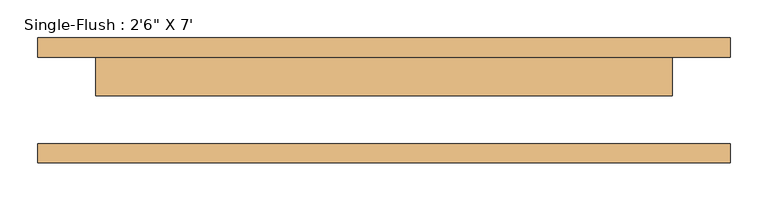
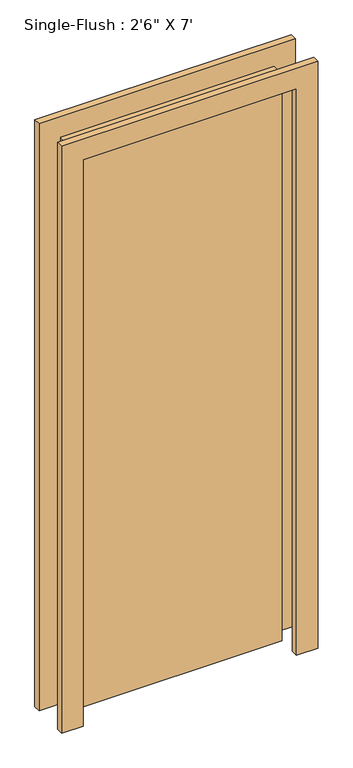
"""IFC4 building model written with IfcOpenShell, lengths in millimetres: door geometry."""

from ifc_helpers import new_model, si_unit, frame, origin, origin_with_axes, place, context, project, spatial, polyline, outline, extrude, source, transform, mapped, element, save


def door_214872d5(model_context):
    return source(origin(), model_context, "Body", "SweptSolid", [
        extrude(outline(polyline([(2209.8, -457.2), (0.0, -457.2), (0.0, -381.0), (2133.6, -381.0), (2133.6, 381.0), (0.0, 381.0), (0.0, 457.2), (2209.8, 457.2), (2209.8, -457.2)])), frame((0.0, 57.15, 0.0), z_axis=(0.0, 1.0, 0.0), x_axis=(0.0, 0.0, 1.0)), (0.0, 0.0, 1.0), 25.4),
        extrude(outline(polyline([(2209.8, 457.2), (2209.8, -457.2), (0.0, -457.2), (0.0, -381.0), (2133.6, -381.0), (2133.6, 381.0), (0.0, 381.0), (0.0, 457.2), (2209.8, 457.2)])), frame((0.0, -82.55, 0.0), z_axis=(0.0, 1.0, 0.0), x_axis=(0.0, 0.0, 1.0)), (0.0, 0.0, 1.0), 25.4),
        extrude(outline(polyline([(381.0, 6.35), (-381.0, 6.35), (-381.0, 57.15), (381.0, 57.15), (381.0, 6.35)])), origin_with_axes(), (0.0, 0.0, 1.0), 2133.6),
    ])


if __name__ == "__main__":
    model = new_model("IFC4")
    model_context = context("Model", 3, world=origin())
    ifc_project = project(units=[si_unit("LENGTHUNIT", "METRE", prefix="MILLI")], contexts=[model_context])
    site = spatial("IfcSite", under=ifc_project)
    building = spatial("IfcBuilding", under=site)
    placement = place(None, origin())
    door_shape = door_214872d5(model_context)
    element("IfcDoor", 1, ObjectType="Single-Flush : 2'6\" X 7'", at=placement, inside=building, context=model_context, shape_type="MappedRepresentation", body=[
        mapped(door_shape, transform((0.0, 0.0, 0.0), x_axis=(1.0, 0.0, 0.0), y_axis=(0.0, 1.0, 0.0), z_axis=(0.0, 0.0, 1.0))),
    ])
    save(model, "model.ifc")

# Revit data of these elements
# Type "Single-Flush : 2'6\" X 7'"
#   Type Mark = "8"
#   Construction Type Id = "MDOOR"
#   Assembly Code = "C1020"
#   Analytic Construction = "Metal"
#   Thickness = 0' - 2"
#   Heat Transfer Coefficient (U) = 0.651978 BTU/(h·ft²·°F)
#   Height = 7' - 0"
#   Trim Projection Ext = 0' - 1"
#   Trim Projection Int = 0' - 1"
#   Trim Width = 0' - 3"
#   Width = 2' - 6"
#   Define Thermal Properties by = 1
#   Door Material = Door - Panel
#   Frame Material = Door - Frame
#   Visual Light Transmittance = 0
#   Solar Heat Gain Coefficient = 0
#   Function = (empty or 0)
#   Wall Closure = (empty or 0)
# Element 1 (IfcDoor, "Single-Flush : 2'6\" X 7'")
#   Materials on its faces: "Door - Frame", "Door - Panel"
# Materials
#   "Door - Panel": class "Wood", colour RGB 210 159 95, transparency 0, Cost = 0
#   "Door - Frame": colour RGB 118 70 51, transparency 0, Cost = 0
